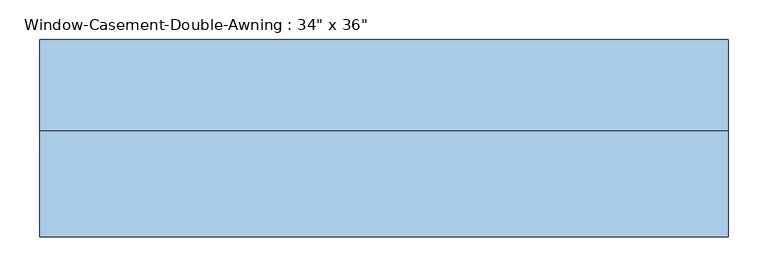
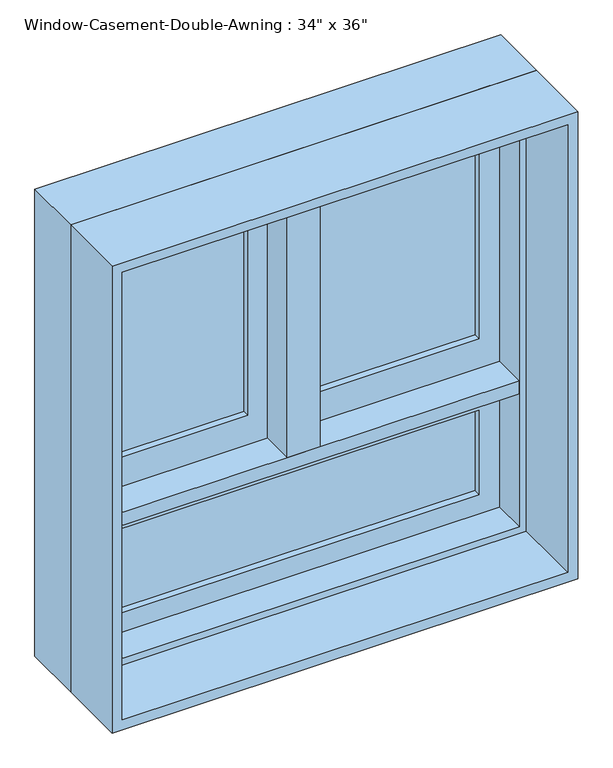
"""IFC4 building model written with IfcOpenShell, lengths in millimetres: window geometry."""

from ifc_helpers import new_model, si_unit, frame, origin, place, context, project, spatial, polyline, outline, extrude, faceted_brep, source, transform, mapped, element, save


def window_ced37e8f(model_context):
    return source(origin(), model_context, "Body", "SolidModel", [
        faceted_brep([(400.05, 82.55, 1797.05), (400.05, 19.05, 1797.05), (-400.05, 19.05, 1797.05), (-400.05, 82.55, 1797.05), (419.1, 133.35, 1816.1), (419.1, 82.55, 1816.1), (-419.1, 82.55, 1816.1), (-419.1, 133.35, 1816.1), (431.8, 19.05, 1828.8), (431.8, 133.35, 1828.8), (-431.8, 133.35, 1828.8), (-431.8, 19.05, 1828.8), (-400.05, 19.05, 946.15), (-400.05, 82.55, 946.15), (-419.1, 82.55, 927.1), (-419.1, 133.35, 927.1), (-431.8, 133.35, 914.4), (-431.8, 19.05, 914.4), (400.05, 19.05, 946.15), (400.05, 82.55, 946.15), (419.1, 82.55, 927.1), (419.1, 133.35, 927.1), (431.8, 133.35, 914.4), (431.8, 19.05, 914.4)], [[[0, 1, 2, 3]], [[4, 5, 6, 7]], [[8, 9, 10, 11]], [[3, 2, 12, 13]], [[7, 6, 14, 15]], [[11, 10, 16, 17]], [[13, 12, 18, 19]], [[15, 14, 20, 21]], [[17, 16, 22, 23]], [[11, 17, 23, 8], [1, 18, 12, 2]], [[19, 18, 1, 0]], [[5, 20, 14, 6], [3, 13, 19, 0]], [[21, 20, 5, 4]], [[23, 22, 9, 8]], [[9, 22, 16, 10], [7, 15, 21, 4]]]),
        extrude(outline(polyline([(1231.9, 419.1), (1816.1, 419.1), (1816.1, 9.525), (1231.9, 9.525), (1231.9, 419.1)]), holes=[polyline([(1289.05, 66.675), (1758.95, 66.675), (1758.95, 361.95), (1289.05, 361.95), (1289.05, 66.675)])]), frame((0.0, 82.55, 0.0), z_axis=(0.0, 1.0, 0.0), x_axis=(0.0, 0.0, 1.0)), (0.0, 0.0, 1.0), 44.45),
        extrude(outline(polyline([(1816.1, -419.1), (1231.9, -419.1), (1231.9, -9.525), (1816.1, -9.525), (1816.1, -419.1)]), holes=[polyline([(1758.95, -66.675), (1289.05, -66.675), (1289.05, -361.95), (1758.95, -361.95), (1758.95, -66.675)])]), frame((0.0, 82.55, 0.0), z_axis=(0.0, 1.0, 0.0), x_axis=(0.0, 0.0, 1.0)), (0.0, 0.0, 1.0), 44.45),
        extrude(outline(polyline([(361.95, 114.3), (361.95, 107.95), (66.675, 107.95), (66.675, 114.3), (361.95, 114.3)])), frame((0.0, 0.0, 1289.05), z_axis=(0.0, 0.0, 1.0), x_axis=(1.0, 0.0, 0.0)), (0.0, 0.0, 1.0), 469.9),
        extrude(outline(polyline([(66.675, 95.25), (66.675, 101.6), (361.95, 101.6), (361.95, 95.25), (66.675, 95.25)])), frame((0.0, 0.0, 1289.05), z_axis=(0.0, 0.0, 1.0), x_axis=(1.0, 0.0, 0.0)), (0.0, 0.0, 1.0), 469.9),
        extrude(outline(polyline([(-66.675, 114.3), (-66.675, 107.95), (-361.95, 107.95), (-361.95, 114.3), (-66.675, 114.3)])), frame((0.0, 0.0, 1289.05), z_axis=(0.0, 0.0, 1.0), x_axis=(1.0, 0.0, 0.0)), (0.0, 0.0, 1.0), 469.9),
        extrude(outline(polyline([(-361.95, 95.25), (-361.95, 101.6), (-66.675, 101.6), (-66.675, 95.25), (-361.95, 95.25)])), frame((0.0, 0.0, 1289.05), z_axis=(0.0, 0.0, 1.0), x_axis=(1.0, 0.0, 0.0)), (0.0, 0.0, 1.0), 469.9),
        extrude(outline(polyline([(400.05, 19.05), (-400.05, 19.05), (-400.05, 82.55), (-419.1, 82.55), (-419.1, 133.35), (419.1, 133.35), (419.1, 82.55), (400.05, 82.55), (400.05, 19.05)])), frame((0.0, 0.0, 1206.5), z_axis=(0.0, 0.0, 1.0), x_axis=(1.0, 0.0, 0.0)), (0.0, 0.0, 1.0), 25.4),
        extrude(outline(polyline([(1206.5, -419.1), (927.1, -419.1), (927.1, 419.1), (1206.5, 419.1), (1206.5, -419.1)]), holes=[polyline([(1149.35, 361.95), (984.25, 361.95), (984.25, -361.95), (1149.35, -361.95), (1149.35, 361.95)])]), frame((0.0, 82.55, 0.0), z_axis=(0.0, 1.0, 0.0), x_axis=(0.0, 0.0, 1.0)), (0.0, 0.0, 1.0), 44.45),
        extrude(outline(polyline([(361.95, 114.3), (361.95, 107.95), (-361.95, 107.95), (-361.95, 114.3), (361.95, 114.3)])), frame((0.0, 0.0, 984.25), z_axis=(0.0, 0.0, 1.0), x_axis=(1.0, 0.0, 0.0)), (0.0, 0.0, 1.0), 165.1),
        extrude(outline(polyline([(361.95, 101.6), (361.95, 95.25), (-361.95, 95.25), (-361.95, 101.6), (361.95, 101.6)])), frame((0.0, 0.0, 984.25), z_axis=(0.0, 0.0, 1.0), x_axis=(1.0, 0.0, 0.0)), (0.0, 0.0, 1.0), 165.1),
        extrude(outline(polyline([(1828.8, -431.8), (914.4, -431.8), (914.4, 431.8), (1828.8, 431.8), (1828.8, -431.8)]), holes=[polyline([(1809.75, 412.75), (933.45, 412.75), (933.45, -412.75), (1809.75, -412.75), (1809.75, 412.75)])]), frame((0.0, -114.3, 0.0), z_axis=(0.0, 1.0, 0.0), x_axis=(0.0, 0.0, 1.0)), (0.0, 0.0, 1.0), 133.35),
        faceted_brep([(9.525, 133.35, 1816.1), (-9.525, 133.35, 1816.1), (-9.525, 82.55, 1816.1), (9.525, 82.55, 1816.1), (9.525, 133.35, 1231.9), (9.525, 82.55, 1231.9), (30.1625, 82.55, 1231.9), (30.1625, 19.05, 1231.9), (-30.1625, 19.05, 1231.9), (-30.1625, 82.55, 1231.9), (-9.525, 82.55, 1231.9), (-9.525, 133.35, 1231.9), (-9.525, 82.55, 1797.05), (-30.1625, 82.55, 1797.05), (-30.1625, 19.05, 1797.05), (30.1625, 19.05, 1797.05), (30.1625, 82.55, 1797.05), (9.525, 82.55, 1797.05)], [[[0, 1, 2, 3]], [[4, 5, 6, 7, 8, 9, 10, 11]], [[1, 0, 4, 11]], [[2, 1, 11, 10, 12]], [[10, 9, 13, 12]], [[9, 8, 14, 13]], [[8, 7, 15, 14]], [[7, 6, 16, 15]], [[6, 5, 17, 16]], [[0, 3, 17, 5, 4]], [[12, 17, 3, 2]], [[17, 12, 13, 14, 15, 16]]]),
    ])


if __name__ == "__main__":
    model = new_model("IFC4")
    model_context = context("Model", 3, world=origin())
    ifc_project = project(units=[si_unit("LENGTHUNIT", "METRE", prefix="MILLI")], contexts=[model_context])
    site = spatial("IfcSite", under=ifc_project)
    building = spatial("IfcBuilding", under=site)
    placement = place(None, origin())
    window_shape = window_ced37e8f(model_context)
    element("IfcWindow", 1, ObjectType="Window-Casement-Double-Awning : 34\" x 36\"", at=placement, inside=building, context=model_context, shape_type="MappedRepresentation", body=[
        mapped(window_shape, transform((0.0, 0.0, 0.0), x_axis=(1.0, 0.0, 0.0), y_axis=(0.0, 1.0, 0.0), z_axis=(0.0, 0.0, 1.0))),
    ])
    save(model, "model.ifc")

# Revit data of these elements
# Type "Window-Casement-Double-Awning : 34\" x 36\""
#   Type Mark = "26"
#   Fire Rating = "0.5h"
#   Assembly Code = "B2020100"
#   Analytic Construction = "Double glazing - domestic"
#   Window Inset [instance default] = 0' - 0"
#   Wall Thickness [instance default] = 0' - 6"
#   Interior Wall Closure [instance default] = 0' - 2 1/4"
#   Half Width = 1' - 5"
#   Visual Light Transmittance = 0.81
#   Thermal Resistance (R) = 1.8146 (h·ft²·°F)/BTU
#   Solar Heat Gain Coefficient = 0.76
#   Rough Width = 2' - 10 1/2"
#   Rough Height = 3' - 0 1/2"
#   Open Window Height = 2' - 0"
#   Height = 3' - 0"
#   Heat Transfer Coefficient (U) = 0.5511 BTU/(h·ft²·°F)
#   Frame Extension [instance default] = 0' - 0 1/4"
#   Exterior Wall Closure [instance default] = 0' - 1 1/4"
#   Awning Height = 1' - 0"
#   Extension Jamb [instance default] = 0' - 2 1/4"
#   Default Sill Height = 3' - 0"
#   Width = 2' - 10"
#   Top Muntin Visibility = yes
#   Interior Trim Visibility [instance default] = yes
#   Bottom Muntin Visibility = yes
#   Exterior Trim Visibility [instance default] = yes
#   Extension Jamb Visibility [instance default] = yes
#   Interior Trim Material = Wood - Stained
#   Muntin Pattern = Muntin Pattern_2x2 : Muntin Pattern_2x2
#   Interior Trim = Trim-Window-Interior-Flat : Picture Frame
#   Interior Frame Material = Wood - Stained
#   Exterior Trim Material = Clad - White
#   Glass Panel Material = Glass
#   Exterior Trim = Trim-Window-Exterior-Flat : with Sill
#   Exterior Frame Material = Clad - White
#   Wall Closure = (empty or 0)
# Element 1 (IfcWindow, "Window-Casement-Double-Awning : 34\" x 36\"")
#   Wall Thickness = 0' - 9"
#   Extension Jamb = 0' - 5 1/4"
#   Materials on its faces: "Wood - Stained", "Glass", "Clad - White"
# Materials
#   "Wood - Stained": class "Wood", colour RGB 224 178 126, transparency 0, Cost = 0
#   "Clad - White": class "Wood", colour RGB 242 242 238, transparency 0, Cost = 0
#   "Glass": class "Glass", colour RGB 0 128 192, transparency 0.75, Description = "Soda Lime Glass", Cost = 0
